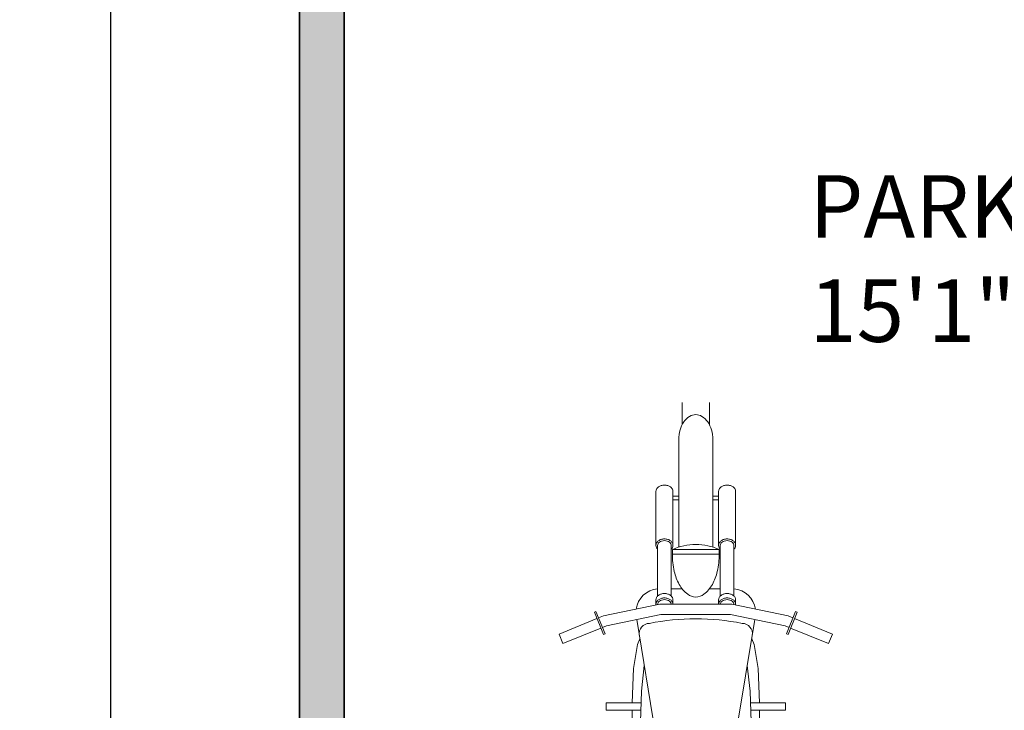
# Model space of a CAD drawing. Units: inches. Extents: x 3008 to 4088, y 1255 to 2137.
# Tile 2 of 30: x 3008 to 3119, y 1462 to 1539. Entities that reach past the tile are written whole.
import ezdxf

# ---------------------------------------------------------------- set-up
doc = ezdxf.new("R2010")
doc.units = ezdxf.units.IN
for name, color, linetype, lineweight in [('A-ANNO-DIMS', 2, 'Continuous', 18), ('A-AREA-IDEN', 7, 'Continuous', 18), ('C-PROP', 1, 'Continuous', 35), ('C-PROP-PATT', 9, 'Continuous', 13), ('C-SITE-VEHC', 9, 'Continuous', 13)]:
    doc.layers.add(name, color=color, linetype=linetype, lineweight=lineweight)
doc.styles.get("Standard").update_dxf_attribs({"font": 'arial.ttf'})
doc.dimstyles.new('ISO-25', dxfattribs={"dimtxt": 8, "dimasz": 2.5, "dimexe": 1.25, "dimexo": 0.625, "dimtad": 1, "dimdec": 1, "dimlunit": 3, "dimtxsty": 'Standard', "dimcen": 2.5, "dimadec": 0, "dimazin": 0, "dimtfac": 1, "dimtdec": 1, "dimtmove": 0, "dimatfit": 3, "dimfxl": 1, "dimarcsym": 0})

# ---------------------------------------------------------------- blocks, each defined once
blk = doc.blocks.new('*D2')
at = {"layer": 'A-ANNO-DIMS', "color": 0, "lineweight": -2, "transparency": 16777216}
for p, q in [((3039.04, 2003.97), (3017.26, 2003.97)), ((3018.51, 2001.47), (3018.51, 1346.47)), ((3039.04, 1343.97), (3017.26, 1343.97))]:
    blk.add_line(p, q, dxfattribs=at)
at = {"layer": 'A-ANNO-DIMS', "color": 0, "transparency": 16777216}
for points in [[(3018.09, 2001.47), (3018.93, 2001.47), (3018.51, 2003.97)], [(3018.09, 1346.47), (3018.93, 1346.47), (3018.51, 1343.97)]]:
    blk.add_solid(points, dxfattribs=at)
at = {"layer": 'Defpoints', "color": 0, "transparency": 16777216}
for p in [(3039.67, 2003.97), (3018.51, 1343.97), (3039.67, 1343.97)]:
    blk.add_point(p, dxfattribs=at)
at = {"layer": 'A-ANNO-DIMS', "color": 0, "transparency": 16777216, "insert": (3013.82, 1673.97), "char_height": 8, "attachment_point": 5, "rotation": 90}
blk.add_mtext("55'", dxfattribs=at)
blk = doc.blocks.new('BIKE')
for p, q in [((34846.04, 15170.344), (34846.04, 15168.869)), ((34847.863, 15170.344), (34847.863, 15168.869)), ((34845.812, 15167.865), (34845.812, 15160.698)), ((34845.812, 15167.865), (34845.812, 15160.698)), ((34848.09, 15167.865), (34848.09, 15160.698)), ((34844.293, 15164.403), (34844.293, 15160.811)), ((34845.432, 15164.403), (34845.432, 15160.811)), ((34845.432, 15164.099), (34845.812, 15164.099)), ((34848.47, 15164.099), (34848.09, 15164.099)), ((34848.47, 15164.403), (34848.47, 15160.811)), ((34849.609, 15164.403), (34849.609, 15160.811)), ((34845.432, 15163.85), (34845.812, 15163.85)), ((34848.47, 15163.85), (34848.09, 15163.85)), ((34844.407, 15160.811), (34844.407, 15157.429)), ((34845.318, 15160.811), (34845.318, 15157.429)), ((34848.584, 15160.811), (34848.584, 15157.429)), ((34849.496, 15160.811), (34849.496, 15157.429)), ((34848.513, 15160.529), (34845.39, 15160.529)), ((34845.39, 15160.235), (34845.39, 15160.529)), ((34845.39, 15160.235), (34845.39, 15160.529)), ((34848.513, 15160.235), (34845.39, 15160.235)), ((34848.513, 15160.235), (34848.513, 15160.529)), ((34845.318, 15157.919), (34846.037, 15157.919)), ((34848.584, 15157.919), (34847.865, 15157.919)), ((34840.801, 15156.108), (34844.559, 15156.882)), ((34844.293, 15156.871), (34844.293, 15157.169)), ((34844.407, 15156.871), (34844.407, 15156.851)), ((34844.559, 15156.882), (34846.951, 15156.882)), ((34845.432, 15156.871), (34845.432, 15157.169)), ((34849.344, 15156.882), (34846.951, 15156.882)), ((34848.47, 15156.871), (34848.47, 15157.169)), ((34853.102, 15156.108), (34849.344, 15156.882)), ((34849.496, 15156.871), (34849.496, 15156.851)), ((34849.609, 15156.871), (34849.609, 15157.169)), ((34840.194, 15156.351), (34840.299, 15156.394)), ((34840.194, 15156.351), (34840.799, 15154.875)), ((34840.299, 15156.394), (34840.905, 15154.919)), ((34840.472, 15155.973), (34840.801, 15156.108)), ((34841.001, 15155.451), (34844.628, 15156.198)), ((34844.628, 15156.198), (34846.951, 15156.198)), ((34849.274, 15156.198), (34846.951, 15156.198)), ((34852.901, 15155.451), (34849.274, 15156.198)), ((34853.603, 15156.394), (34852.998, 15154.919)), ((34853.43, 15155.973), (34853.102, 15156.108)), ((34853.709, 15156.351), (34853.103, 15154.875)), ((34853.709, 15156.351), (34853.603, 15156.394)), ((34837.837, 15154.891), (34840.367, 15155.929)), ((34840.732, 15155.34), (34841.001, 15155.451)), ((34844.855, 15144.722), (34843.012, 15155.865)), ((34849.048, 15144.722), (34850.89, 15155.865)), ((34853.171, 15155.34), (34852.901, 15155.451)), ((34856.065, 15154.891), (34853.536, 15155.929)), ((34837.837, 15154.891), (34838.097, 15154.259)), ((34838.097, 15154.259), (34840.626, 15155.297)), ((34840.799, 15154.875), (34840.905, 15154.919)), ((34853.103, 15154.875), (34852.998, 15154.919)), ((34855.805, 15154.259), (34853.276, 15155.297)), ((34856.065, 15154.891), (34855.805, 15154.259)), ((34842.804, 15152.592), (34843.061, 15154.2)), ((34843.061, 15154.2), (34843.225, 15154.581)), ((34850.842, 15154.2), (34850.678, 15154.581)), ((34851.099, 15152.592), (34850.842, 15154.2)), ((34842.703, 15150.307), (34842.804, 15152.592)), ((34843.328, 15151.093), (34843.52, 15152.795)), ((34850.574, 15151.093), (34850.383, 15152.795)), ((34851.199, 15150.307), (34851.099, 15152.592)), ((34843.23, 15147.751), (34843.328, 15151.093)), ((34850.673, 15147.751), (34850.574, 15151.093)), ((34840.971, 15150.307), (34843.305, 15150.307)), ((34840.971, 15149.813), (34840.971, 15150.307)), ((34852.932, 15150.307), (34850.598, 15150.307)), ((34852.932, 15149.813), (34852.932, 15150.307)), ((34843.29, 15149.813), (34840.971, 15149.813)), ((34842.703, 15144.873), (34842.703, 15149.813)), ((34850.612, 15149.813), (34852.932, 15149.813)), ((34851.199, 15144.873), (34851.199, 15149.813)), ((34843.23, 15144.145), (34843.23, 15147.751)), ((34850.673, 15144.145), (34850.673, 15147.751)), ((34842.703, 15144.873), (34842.248, 15142.195)), ((34842.703, 15144.873), (34843.23, 15144.873)), ((34847.846, 15144.636), (34846.057, 15144.636)), ((34851.199, 15144.873), (34850.673, 15144.873)), ((34851.199, 15144.873), (34851.655, 15142.195)), ((34844.464, 15143.561), (34843.601, 15128.195)), ((34843.854, 15143.464), (34844.07, 15142.195)), ((34843.913, 15143.462), (34844.458, 15143.462)), ((34849.439, 15143.561), (34850.301, 15128.195)), ((34849.989, 15143.462), (34849.444, 15143.462)), ((34850.048, 15143.464), (34849.832, 15142.195)), ((34842.248, 15142.195), (34844.07, 15142.195)), ((34842.248, 15137.821), (34842.248, 15142.195)), ((34844.07, 15137.821), (34844.07, 15142.195)), ((34851.655, 15142.195), (34849.832, 15142.195)), ((34849.832, 15137.821), (34849.832, 15142.195)), ((34851.655, 15137.821), (34851.655, 15142.195)), ((34841.794, 15137.821), (34844.142, 15137.821)), ((34841.794, 15137.328), (34841.794, 15137.821)), ((34852.108, 15137.821), (34849.761, 15137.821)), ((34852.108, 15137.328), (34852.108, 15137.821)), ((34844.114, 15137.328), (34841.794, 15137.328)), ((34842.248, 15127.566), (34842.248, 15137.328)), ((34844.07, 15136.554), (34844.07, 15137.328)), ((34849.789, 15137.328), (34852.108, 15137.328)), ((34849.832, 15136.554), (34849.832, 15137.328)), ((34851.655, 15127.566), (34851.655, 15137.328)), ((34842.248, 15127.566), (34843.75, 15127.566)), ((34842.248, 15127.566), (34842.476, 15126.269)), ((34844.015, 15127.251), (34843.843, 15126.269)), ((34849.887, 15127.251), (34850.06, 15126.269)), ((34851.655, 15127.566), (34850.153, 15127.566)), ((34851.655, 15127.566), (34851.427, 15126.269)), ((34849.164, 15126.992), (34844.739, 15126.992)), ((34845.47, 15126.992), (34845.47, 15126.882)), ((34845.812, 15126.992), (34845.812, 15126.882)), ((34848.09, 15126.992), (34848.09, 15126.882)), ((34848.432, 15126.992), (34848.432, 15126.882)), ((34842.476, 15126.269), (34843.843, 15126.269)), ((34845.812, 15126.29), (34845.812, 15124.029)), ((34847.749, 15126.54), (34846.154, 15126.54)), ((34847.749, 15126.198), (34846.154, 15126.198)), ((34848.09, 15126.29), (34848.09, 15124.029)), ((34851.427, 15126.269), (34850.06, 15126.269)), ((34846.291, 15123.822), (34846.291, 15124.661)), ((34846.291, 15124.661), (34847.611, 15124.661)), ((34847.611, 15124.661), (34847.611, 15123.822)), ((34846.291, 15124.547), (34847.611, 15124.547)), ((34847.611, 15123.822), (34846.291, 15123.822))]:
    blk.add_line(p, q)
for points in [[(34845.812, 15167.865, -0.068977), (34845.904, 15168.528, -0.081012), (34846.146, 15169.045, -0.107014), (34846.54, 15169.419, -0.137239), (34846.951, 15169.534, -0.137239), (34847.362, 15169.419, -0.107014), (34847.757, 15169.045, -0.081012), (34847.999, 15168.528, -0.068977), (34848.09, 15167.865, -0.068977)], [(34845.432, 15164.403, 0.125099), (34845.392, 15164.563, 0.105827), (34845.265, 15164.71, 0.086577), (34845.087, 15164.802, 0.0766), (34844.863, 15164.837, 0.0766), (34844.638, 15164.802, 0.086577), (34844.46, 15164.71, 0.105827), (34844.334, 15164.563, 0.125099), (34844.293, 15164.403, 0.125099)], [(34848.47, 15164.403, -0.125099), (34848.511, 15164.563, -0.105827), (34848.637, 15164.71, -0.086577), (34848.816, 15164.802, -0.0766), (34849.04, 15164.837, -0.0766), (34849.264, 15164.802, -0.086577), (34849.443, 15164.71, -0.105827), (34849.569, 15164.563, -0.125099), (34849.609, 15164.403, -0.125099)], [(34845.318, 15160.551, 0.067261), (34845.392, 15160.652, 0.125099), (34845.432, 15160.811, 0.125099), (34845.392, 15160.971, 0.105827), (34845.265, 15161.118, 0.086577), (34845.087, 15161.211, 0.0766), (34844.863, 15161.245, 0.0766), (34844.638, 15161.211, 0.086577), (34844.46, 15161.118, 0.105827), (34844.334, 15160.971, 0.125099), (34844.293, 15160.811, 0.125099)], [(34844.293, 15160.811, 0.125099), (34844.334, 15160.652, 0.067261), (34844.407, 15160.551, 0.086577)], [(34845.318, 15160.811, 0.125099), (34845.292, 15160.917, 0.105827), (34845.196, 15161.028, 0.086577), (34845.053, 15161.102, 0.0766), (34844.863, 15161.132, 0.0766), (34844.673, 15161.102, 0.086577), (34844.529, 15161.028, 0.105827), (34844.434, 15160.917, 0.125099), (34844.407, 15160.811, 0.125099)], [(34848.584, 15160.551, -0.067261), (34848.511, 15160.652, -0.125099), (34848.47, 15160.811, -0.125099), (34848.511, 15160.971, -0.105827), (34848.637, 15161.118, -0.086577), (34848.816, 15161.211, -0.0766), (34849.04, 15161.245, -0.0766), (34849.264, 15161.211, -0.086577), (34849.443, 15161.118, -0.105827), (34849.569, 15160.971, -0.125099), (34849.609, 15160.811, -0.125099)], [(34848.584, 15160.811, -0.125099), (34848.611, 15160.917, -0.105827), (34848.706, 15161.028, -0.086577), (34848.85, 15161.102, -0.0766), (34849.04, 15161.132, -0.0766), (34849.23, 15161.102, -0.086577), (34849.374, 15161.028, -0.105827), (34849.469, 15160.917, -0.125099), (34849.496, 15160.811, -0.125099)], [(34849.609, 15160.811, -0.125099), (34849.569, 15160.652, -0.067261), (34849.496, 15160.551, -0.086577)], [(34846.951, 15157.368, -0.163989), (34846.412, 15157.55, -0.105862), (34845.847, 15158.208, -0.069323), (34845.519, 15159.08, -0.055531), (34845.39, 15160.235, -0.055531)], [(34848.513, 15160.235, -0.055531), (34848.384, 15159.08, -0.069323), (34848.055, 15158.208, -0.105862), (34847.49, 15157.55, -0.163989), (34846.951, 15157.368, -0.163989)], [(34845.432, 15157.169, 0.125099), (34845.392, 15157.329, 0.105827), (34845.265, 15157.476, 0.086577), (34845.087, 15157.568, 0.0766), (34844.863, 15157.603, 0.0766), (34844.638, 15157.568, 0.086577), (34844.46, 15157.476, 0.105827), (34844.334, 15157.329, 0.125099), (34844.293, 15157.169, 0.125099)], [(34848.47, 15157.169, -0.125099), (34848.511, 15157.329, -0.105827), (34848.637, 15157.476, -0.086577), (34848.816, 15157.568, -0.0766), (34849.04, 15157.603, -0.0766), (34849.264, 15157.568, -0.086577), (34849.443, 15157.476, -0.105827), (34849.569, 15157.329, -0.125099), (34849.609, 15157.169, -0.125099)], [(34845.432, 15156.882, 0.117252), (34845.392, 15157.031, 0.105827), (34845.265, 15157.178, 0.086577), (34845.087, 15157.271, 0.0766), (34844.863, 15157.306, 0.0766), (34844.638, 15157.271, 0.086577), (34844.46, 15157.178, 0.105827), (34844.334, 15157.031, 0.125099), (34844.293, 15156.871, 0.125099)], [(34844.293, 15156.871, 0.032819), (34844.296, 15156.828, 0.067261)], [(34845.318, 15156.882, 0.113202), (34845.292, 15156.977, 0.105827), (34845.196, 15157.088, 0.086577), (34845.053, 15157.162, 0.0766), (34844.863, 15157.192, 0.0766), (34844.673, 15157.162, 0.086577), (34844.529, 15157.088, 0.105827), (34844.434, 15156.977, 0.125099), (34844.407, 15156.871, 0.125099)], [(34848.47, 15156.882, -0.117252), (34848.511, 15157.031, -0.105827), (34848.637, 15157.178, -0.086577), (34848.816, 15157.271, -0.0766), (34849.04, 15157.306, -0.0766), (34849.264, 15157.271, -0.086577), (34849.443, 15157.178, -0.105827), (34849.569, 15157.031, -0.125099), (34849.609, 15156.871, -0.125099)], [(34848.584, 15156.882, -0.113202), (34848.611, 15156.977, -0.105827), (34848.706, 15157.088, -0.086577), (34848.85, 15157.162, -0.0766), (34849.04, 15157.192, -0.0766), (34849.23, 15157.162, -0.086577), (34849.374, 15157.088, -0.105827), (34849.469, 15156.977, -0.125099), (34849.496, 15156.871, -0.125099)], [(34849.609, 15156.871, -0.032819), (34849.607, 15156.828, -0.067261)]]:
    blk.add_lwpolyline(points, format="xyb")
for centre, radius, start, end in [((34846.951, 15157.242), 3.638, 64.58823, 115.41177), ((34844.552, 15156.324), 1.595, 95.22072, 171.67796), ((34849.35, 15156.324), 1.595, 8.32204, 84.77928), ((34843.861, 15154.923), 0.684, 90, 189.38978), ((34846.951, 15140.123), 15.789, 78.71287, 101.28713), ((34850.042, 15154.923), 0.684, 350.61022, 90), ((34846.003, 15142.998), 1.639, 88.11253, 159.92642), ((34845.529, 15144.833), 0.684, 189.38978, 226.48769), ((34847.9, 15142.998), 1.639, 20.07358, 91.88747), ((34848.373, 15144.833), 0.684, 313.51231, 350.61022), ((34843.913, 15144.145), 0.684, 180, 270), ((34849.989, 15144.145), 0.684, 270, 0), ((34844.739, 15128.131), 1.139, 176.78649, 270), ((34849.164, 15128.131), 1.139, 270, 3.21351), ((34846.154, 15126.882), 0.684, 180, 270), ((34846.154, 15126.882), 0.342, 180, 270), ((34847.749, 15126.882), 0.684, 270, 0), ((34847.749, 15126.882), 0.342, 270, 0), ((34846.951, 15124.029), 1.139, 180, 0)]:
    blk.add_arc(centre, radius, start, end)

msp = doc.modelspace()

# ---------------------------------------------------------------- hatches: boundary and pattern name
at = {"layer": 'C-PROP-PATT'}
h = msp.add_hatch(color=256, dxfattribs=at)
h.dxf.hatch_style = 1
h.paths.add_polyline_path([(3519.67, 2003.97), (3039.67, 2003.97), (3039.67, 1343.97), (3051.67, 1343.97), (3051.67, 1348.97), (3044.67, 1348.97), (3044.67, 1998.97), (3514.67, 1998.97), (3514.67, 1348.97), (3219.67, 1348.97), (3219.67, 1343.97), (3519.67, 1343.97)])

# ---------------------------------------------------------------- linework, layer by layer
at = {"layer": 'C-PROP'}
for p, q in [((3039.67, 1343.97), (3039.67, 2003.97)), ((3044.67, 1348.97), (3044.67, 1998.97))]:
    msp.add_line(p, q, dxfattribs=at)

# ---------------------------------------------------------------- block references
at = {"layer": 'C-SITE-VEHC', "xscale": 1.67889555227424, "yscale": 1.67889555227424, "zscale": 1.67889555227424}
msp.add_blockref('BIKE', (-55420.37, -23973.42), dxfattribs=at)

# ---------------------------------------------------------------- texts
at = {"layer": 'A-AREA-IDEN', "insert": (3096.73, 1521.46), "char_height": 7, "attachment_point": 1}
msp.add_mtext_dynamic_manual_height_columns('{\\fTimes New Roman|b0|i0|c0|p18;PARKING\\P15\'1"X16\'0"}', width=105.6127, gutter_width=12.5, heights=[0], dxfattribs=at)

# ---------------------------------------------------------------- dimensions: what is measured, and where the dimension line sits
at = {"layer": 'A-ANNO-DIMS'}
dim = msp.add_linear_dim(base=(3018.51, 1343.97), p1=(3039.67, 2003.97), p2=(3039.67, 1343.97), angle=90, dimstyle='ISO-25', override={"dimclrd": 0, "dimclre": 0, "dimclrt": 0}, dxfattribs=at)
dim.commit()
dim.dimension.update_dxf_attribs({"geometry": '*D2', "text_midpoint": (3013.82, 1673.97)})

doc.saveas('drawing.dxf')
